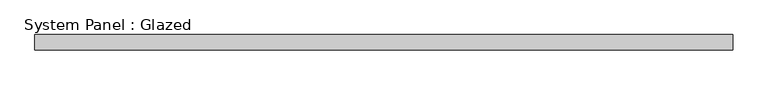
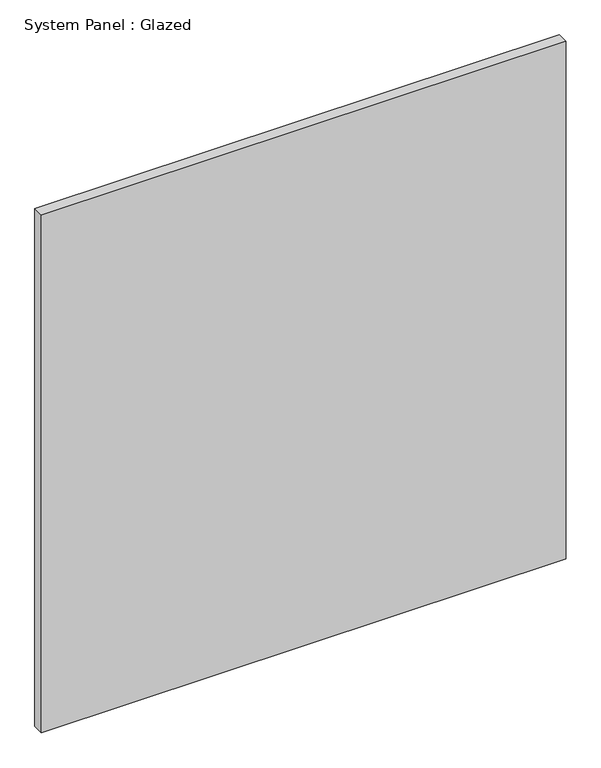
"""IFC4 building model written with IfcOpenShell, lengths in millimetres: plate geometry, System Panel : Glazed."""

from ifc_helpers import new_model, si_unit, origin, origin_with_axes, place, context, project, spatial, polyline, outline, extrude, source, transform, mapped, element, save


def system_panel_glazed_7acd6de3(model_context):
    return source(origin(), model_context, "Body", "SweptSolid", [
        extrude(outline(polyline([(584.2, 19.05), (-584.2, 19.05), (-584.2, 44.45), (584.2, 44.45), (584.2, 19.05)])), origin_with_axes(), (0.0, 0.0, 1.0), 1219.2),
    ])


if __name__ == "__main__":
    model = new_model("IFC4")
    model_context = context("Model", 3, world=origin())
    ifc_project = project(units=[si_unit("LENGTHUNIT", "METRE", prefix="MILLI")], contexts=[model_context])
    site = spatial("IfcSite", under=ifc_project)
    building = spatial("IfcBuilding", under=site)
    placement = place(None, origin())
    system_panel_glazed_shape = system_panel_glazed_7acd6de3(model_context)
    element("IfcPlate", 1, ObjectType="System Panel : Glazed", at=placement, inside=building, context=model_context, shape_type="MappedRepresentation", body=[
        mapped(system_panel_glazed_shape, transform((0.0, 0.0, 0.0), x_axis=(1.0, 0.0, 0.0), y_axis=(0.0, 1.0, 0.0), z_axis=(0.0, 0.0, 1.0))),
    ])
    save(model, "model.ifc")

# Revit data of these elements
# Type "System Panel : Glazed"
#   Construction Type Id = "GSP4R"
#   Analytic Construction = "1/8 in Pilkington single glazing"
#   Visual Light Transmittance = 0.9
#   Solar Heat Gain Coefficient = 0.86
#   Heat Transfer Coefficient (U) = 1.18115 BTU/(h·ft²·°F)
# Element 1 (IfcPlate, "System Panel : Glazed")
#   Materials on its faces: "Glass"
# Materials
#   "Glass": class "Glass", colour RGB 0 128 192, transparency 0.75, Description = "Soda Lime Glass", Cost = 0
